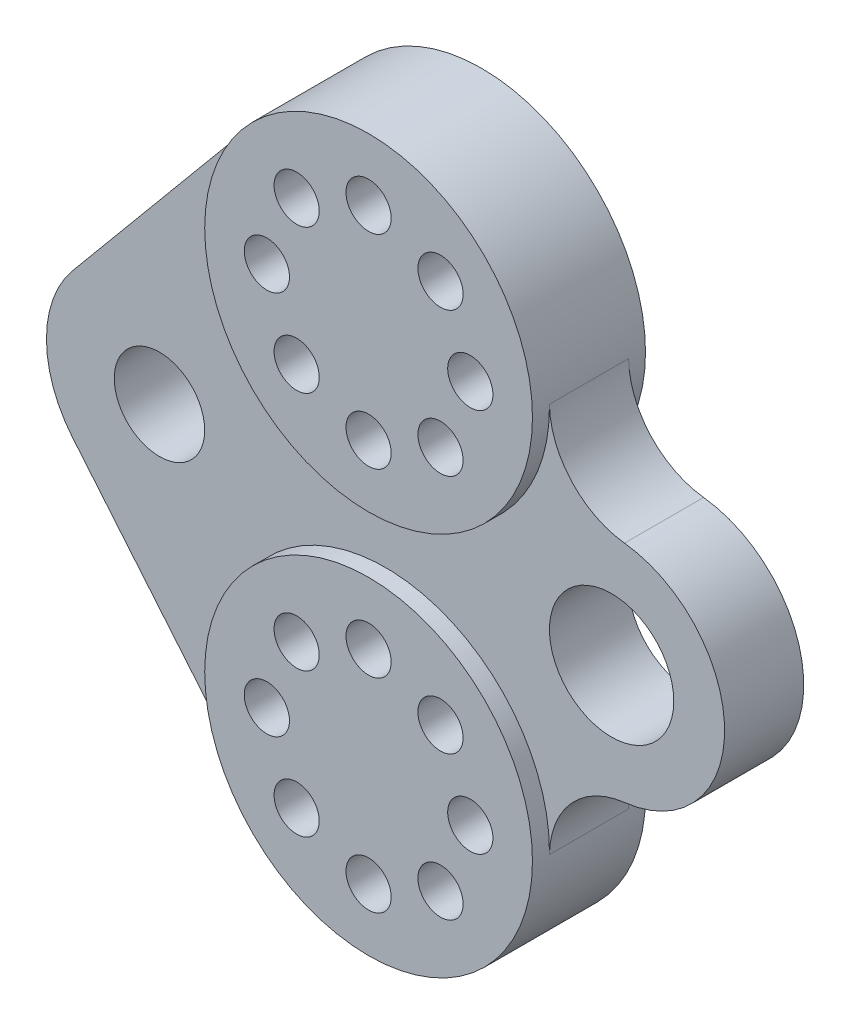
ISO-10303-21;
HEADER;
FILE_DESCRIPTION(('STEP AP214'),'2;1');
FILE_NAME('part.step','',(''),(''),'','','');
FILE_SCHEMA(('AUTOMOTIVE_DESIGN { 1 0 10303 214 1 1 1 1 }'));
ENDSEC;
DATA;
#1=APPLICATION_CONTEXT('core data for automotive mechanical design processes');
#2=APPLICATION_PROTOCOL_DEFINITION('international standard','automotive_design',2000,#1);
#3=PRODUCT_CONTEXT('',#1,'mechanical');
#4=PRODUCT('Part','Part','',(#3));
#5=PRODUCT_RELATED_PRODUCT_CATEGORY('part','',(#4));
#6=PRODUCT_DEFINITION_FORMATION('','',#4);
#7=PRODUCT_DEFINITION_CONTEXT('part definition',#1,'design');
#8=PRODUCT_DEFINITION('design','',#6,#7);
#9=PRODUCT_DEFINITION_SHAPE('','',#8);
#10=(LENGTH_UNIT() NAMED_UNIT(*) SI_UNIT(.MILLI.,.METRE.));
#11=(NAMED_UNIT(*) PLANE_ANGLE_UNIT() SI_UNIT($,.RADIAN.));
#12=(NAMED_UNIT(*) SI_UNIT($,.STERADIAN.) SOLID_ANGLE_UNIT());
#13=UNCERTAINTY_MEASURE_WITH_UNIT(LENGTH_MEASURE(1.E-05),#10,'distance_accuracy_value','');
#14=(GEOMETRIC_REPRESENTATION_CONTEXT(3) GLOBAL_UNCERTAINTY_ASSIGNED_CONTEXT((#13)) GLOBAL_UNIT_ASSIGNED_CONTEXT((#10,
#11,#12)) REPRESENTATION_CONTEXT('',''));
#15=CARTESIAN_POINT('',(0.,0.,0.));
#16=DIRECTION('',(0.,0.,1.));
#17=DIRECTION('',(1.,0.,0.));
#18=AXIS2_PLACEMENT_3D('',#15,#16,#17);
#19=CARTESIAN_POINT('',(-40.,-34.,7.));
#20=DIRECTION('',(0.,0.,1.));
#21=DIRECTION('',(1.,0.,0.));
#22=AXIS2_PLACEMENT_3D('',#19,#20,#21);
#23=PLANE('',#22);
#24=CARTESIAN_POINT('',(-40.,-34.,7.));
#25=DIRECTION('',(0.,0.,1.));
#26=DIRECTION('',(1.,0.,0.));
#27=AXIS2_PLACEMENT_3D('',#24,#25,#26);
#28=CIRCLE('',#27,8.00000000000001);
#29=CARTESIAN_POINT('',(-32.,-34.,7.));
#30=VERTEX_POINT('',#29);
#31=EDGE_CURVE('E141',#30,#30,#28,.T.);
#32=ORIENTED_EDGE('',*,*,#31,.F.);
#33=EDGE_LOOP('',(#32));
#34=FACE_BOUND('',#33,.T.);
#35=DIRECTION('',(0.639628478431684,-0.768684206666931,0.));
#36=VECTOR('',#35,1.);
#37=CARTESIAN_POINT('',(-55.3736841333386,-46.7925695686337,7.));
#38=LINE('',#37,#36);
#39=CARTESIAN_POINT('',(-55.3736841333386,-46.7925695686337,7.));
#40=VERTEX_POINT('',#39);
#41=CARTESIAN_POINT('',(-22.291841993341,-86.5492258745188,7.));
#42=VERTEX_POINT('',#41);
#43=EDGE_CURVE('E99',#40,#42,#38,.T.);
#44=ORIENTED_EDGE('',*,*,#43,.T.);
#45=CARTESIAN_POINT('',(0.,-68.,7.));
#46=DIRECTION('',(0.,0.,1.));
#47=DIRECTION('',(1.,0.,0.));
#48=AXIS2_PLACEMENT_3D('',#45,#46,#47);
#49=CIRCLE('',#48,29.);
#50=CARTESIAN_POINT('',(28.9955422378425,-68.5084587824885,7.));
#51=VERTEX_POINT('',#50);
#52=EDGE_CURVE('E168',#42,#51,#49,.F.);
#53=ORIENTED_EDGE('',*,*,#52,.T.);
#54=CARTESIAN_POINT('',(43.9932364987956,-68.7714547044654,7.));
#55=DIRECTION('',(0.,0.,-1.));
#56=DIRECTION('',(-1.,0.,0.));
#57=AXIS2_PLACEMENT_3D('',#54,#55,#56);
#58=CIRCLE('',#57,15.);
#59=CARTESIAN_POINT('',(42.2818494278832,-53.8694026882659,7.));
#60=VERTEX_POINT('',#59);
#61=EDGE_CURVE('E120',#51,#60,#58,.T.);
#62=ORIENTED_EDGE('',*,*,#61,.T.);
#63=CARTESIAN_POINT('',(40.,-34.,7.));
#64=DIRECTION('',(0.,0.,1.));
#65=DIRECTION('',(1.,0.,0.));
#66=AXIS2_PLACEMENT_3D('',#63,#64,#65);
#67=CIRCLE('',#66,20.);
#68=CARTESIAN_POINT('',(42.2818494278832,-14.1305973117341,7.));
#69=VERTEX_POINT('',#68);
#70=EDGE_CURVE('E112',#60,#69,#67,.T.);
#71=ORIENTED_EDGE('',*,*,#70,.T.);
#72=CARTESIAN_POINT('',(43.9932364987956,0.771454704465369,7.));
#73=DIRECTION('',(0.,0.,-1.));
#74=DIRECTION('',(1.,0.,0.));
#75=AXIS2_PLACEMENT_3D('',#72,#73,#74);
#76=CIRCLE('',#75,15.);
#77=CARTESIAN_POINT('',(28.9955422378425,0.508458782488539,7.));
#78=VERTEX_POINT('',#77);
#79=EDGE_CURVE('E113',#69,#78,#76,.T.);
#80=ORIENTED_EDGE('',*,*,#79,.T.);
#81=CARTESIAN_POINT('',(0.,0.,7.));
#82=DIRECTION('',(0.,0.,1.));
#83=DIRECTION('',(1.,0.,0.));
#84=AXIS2_PLACEMENT_3D('',#81,#82,#83);
#85=CIRCLE('',#84,29.);
#86=CARTESIAN_POINT('',(-22.291841993341,18.5492258745188,7.));
#87=VERTEX_POINT('',#86);
#88=EDGE_CURVE('E195',#78,#87,#85,.F.);
#89=ORIENTED_EDGE('',*,*,#88,.T.);
#90=DIRECTION('',(-0.639628478431684,-0.768684206666931,0.));
#91=VECTOR('',#90,1.);
#92=CARTESIAN_POINT('',(-55.3736841333386,-21.2074304313663,7.));
#93=LINE('',#92,#91);
#94=CARTESIAN_POINT('',(-55.3736841333386,-21.2074304313663,7.));
#95=VERTEX_POINT('',#94);
#96=EDGE_CURVE('E61',#87,#95,#93,.T.);
#97=ORIENTED_EDGE('',*,*,#96,.T.);
#98=CARTESIAN_POINT('',(-40.,-34.,7.));
#99=DIRECTION('',(0.,0.,1.));
#100=DIRECTION('',(1.,0.,0.));
#101=AXIS2_PLACEMENT_3D('',#98,#99,#100);
#102=CIRCLE('',#101,20.);
#103=EDGE_CURVE('E155',#95,#40,#102,.T.);
#104=ORIENTED_EDGE('',*,*,#103,.T.);
#105=EDGE_LOOP('',(#44,#53,#62,#71,#80,#89,#97,#104));
#106=FACE_BOUND('',#105,.T.);
#107=CARTESIAN_POINT('',(40.,-34.,7.));
#108=DIRECTION('',(0.,0.,1.));
#109=DIRECTION('',(1.,0.,0.));
#110=AXIS2_PLACEMENT_3D('',#107,#108,#109);
#111=CIRCLE('',#110,11.);
#112=CARTESIAN_POINT('',(51.,-34.,7.));
#113=VERTEX_POINT('',#112);
#114=EDGE_CURVE('E189',#113,#113,#111,.T.);
#115=ORIENTED_EDGE('',*,*,#114,.F.);
#116=EDGE_LOOP('',(#115));
#117=FACE_BOUND('',#116,.T.);
#118=ADVANCED_FACE('F44',(#34,#106,#117),#23,.T.);
#119=CARTESIAN_POINT('',(-40.,-34.,-7.));
#120=DIRECTION('',(0.,0.,1.));
#121=DIRECTION('',(1.,0.,0.));
#122=AXIS2_PLACEMENT_3D('',#119,#120,#121);
#123=PLANE('',#122);
#124=CARTESIAN_POINT('',(0.,-68.,-7.));
#125=DIRECTION('',(0.,0.,1.));
#126=DIRECTION('',(1.,0.,0.));
#127=AXIS2_PLACEMENT_3D('',#124,#125,#126);
#128=CIRCLE('',#127,29.);
#129=CARTESIAN_POINT('',(-22.291841993341,-86.5492258745188,-7.));
#130=VERTEX_POINT('',#129);
#131=CARTESIAN_POINT('',(28.9955422378425,-68.5084587824885,-7.));
#132=VERTEX_POINT('',#131);
#133=EDGE_CURVE('E169',#130,#132,#128,.F.);
#134=ORIENTED_EDGE('',*,*,#133,.F.);
#135=DIRECTION('',(0.639628478431684,-0.768684206666931,0.));
#136=VECTOR('',#135,1.);
#137=CARTESIAN_POINT('',(-55.3736841333386,-46.7925695686337,-7.));
#138=LINE('',#137,#136);
#139=CARTESIAN_POINT('',(-55.3736841333386,-46.7925695686337,-7.));
#140=VERTEX_POINT('',#139);
#141=EDGE_CURVE('E142',#140,#130,#138,.T.);
#142=ORIENTED_EDGE('',*,*,#141,.F.);
#143=CARTESIAN_POINT('',(-40.,-34.,-7.));
#144=DIRECTION('',(0.,0.,1.));
#145=DIRECTION('',(1.,0.,0.));
#146=AXIS2_PLACEMENT_3D('',#143,#144,#145);
#147=CIRCLE('',#146,20.);
#148=CARTESIAN_POINT('',(-55.3736841333386,-21.2074304313663,-7.));
#149=VERTEX_POINT('',#148);
#150=EDGE_CURVE('E139',#149,#140,#147,.T.);
#151=ORIENTED_EDGE('',*,*,#150,.F.);
#152=DIRECTION('',(-0.639628478431684,-0.768684206666931,0.));
#153=VECTOR('',#152,1.);
#154=CARTESIAN_POINT('',(-55.3736841333386,-21.2074304313663,-7.));
#155=LINE('',#154,#153);
#156=CARTESIAN_POINT('',(-22.291841993341,18.5492258745188,-7.));
#157=VERTEX_POINT('',#156);
#158=EDGE_CURVE('E95',#157,#149,#155,.T.);
#159=ORIENTED_EDGE('',*,*,#158,.F.);
#160=CARTESIAN_POINT('',(0.,0.,-7.));
#161=DIRECTION('',(0.,0.,1.));
#162=DIRECTION('',(1.,0.,0.));
#163=AXIS2_PLACEMENT_3D('',#160,#161,#162);
#164=CIRCLE('',#163,29.);
#165=CARTESIAN_POINT('',(28.9955422378425,0.508458782488539,-7.));
#166=VERTEX_POINT('',#165);
#167=EDGE_CURVE('E88',#166,#157,#164,.F.);
#168=ORIENTED_EDGE('',*,*,#167,.F.);
#169=CARTESIAN_POINT('',(43.9932364987956,0.771454704465369,-7.));
#170=DIRECTION('',(0.,0.,-1.));
#171=DIRECTION('',(1.,0.,0.));
#172=AXIS2_PLACEMENT_3D('',#169,#170,#171);
#173=CIRCLE('',#172,15.);
#174=CARTESIAN_POINT('',(42.2818494278832,-14.1305973117341,-7.));
#175=VERTEX_POINT('',#174);
#176=EDGE_CURVE('E149',#175,#166,#173,.T.);
#177=ORIENTED_EDGE('',*,*,#176,.F.);
#178=CARTESIAN_POINT('',(40.,-34.,-7.));
#179=DIRECTION('',(0.,0.,1.));
#180=DIRECTION('',(1.,0.,0.));
#181=AXIS2_PLACEMENT_3D('',#178,#179,#180);
#182=CIRCLE('',#181,20.);
#183=CARTESIAN_POINT('',(42.2818494278832,-53.8694026882659,-7.));
#184=VERTEX_POINT('',#183);
#185=EDGE_CURVE('E130',#184,#175,#182,.T.);
#186=ORIENTED_EDGE('',*,*,#185,.F.);
#187=CARTESIAN_POINT('',(43.9932364987956,-68.7714547044654,-7.));
#188=DIRECTION('',(0.,0.,-1.));
#189=DIRECTION('',(-1.,0.,0.));
#190=AXIS2_PLACEMENT_3D('',#187,#188,#189);
#191=CIRCLE('',#190,15.);
#192=EDGE_CURVE('E148',#132,#184,#191,.T.);
#193=ORIENTED_EDGE('',*,*,#192,.F.);
#194=EDGE_LOOP('',(#134,#142,#151,#159,#168,#177,#186,#193));
#195=FACE_BOUND('',#194,.T.);
#196=CARTESIAN_POINT('',(-40.,-34.,-7.));
#197=DIRECTION('',(0.,0.,1.));
#198=DIRECTION('',(1.,0.,0.));
#199=AXIS2_PLACEMENT_3D('',#196,#197,#198);
#200=CIRCLE('',#199,8.00000000000001);
#201=CARTESIAN_POINT('',(-32.,-34.,-7.));
#202=VERTEX_POINT('',#201);
#203=EDGE_CURVE('E181',#202,#202,#200,.T.);
#204=ORIENTED_EDGE('',*,*,#203,.T.);
#205=EDGE_LOOP('',(#204));
#206=FACE_BOUND('',#205,.T.);
#207=CARTESIAN_POINT('',(40.,-34.,-7.));
#208=DIRECTION('',(0.,0.,1.));
#209=DIRECTION('',(1.,0.,0.));
#210=AXIS2_PLACEMENT_3D('',#207,#208,#209);
#211=CIRCLE('',#210,11.);
#212=CARTESIAN_POINT('',(51.,-34.,-7.));
#213=VERTEX_POINT('',#212);
#214=EDGE_CURVE('E188',#213,#213,#211,.T.);
#215=ORIENTED_EDGE('',*,*,#214,.T.);
#216=EDGE_LOOP('',(#215));
#217=FACE_BOUND('',#216,.T.);
#218=ADVANCED_FACE('F178',(#195,#206,#217),#123,.F.);
#219=CARTESIAN_POINT('',(-40.,-34.,7.));
#220=DIRECTION('',(0.,0.,-1.));
#221=DIRECTION('',(-1.,0.,0.));
#222=AXIS2_PLACEMENT_3D('',#219,#220,#221);
#223=CYLINDRICAL_SURFACE('',#222,20.);
#224=ORIENTED_EDGE('',*,*,#150,.T.);
#225=DIRECTION('',(0.,0.,-1.));
#226=VECTOR('',#225,1.);
#227=CARTESIAN_POINT('',(-55.3736841333386,-46.7925695686337,7.));
#228=LINE('',#227,#226);
#229=EDGE_CURVE('E11',#40,#140,#228,.T.);
#230=ORIENTED_EDGE('',*,*,#229,.F.);
#231=ORIENTED_EDGE('',*,*,#103,.F.);
#232=DIRECTION('',(0.,0.,-1.));
#233=VECTOR('',#232,1.);
#234=CARTESIAN_POINT('',(-55.3736841333386,-21.2074304313663,7.));
#235=LINE('',#234,#233);
#236=EDGE_CURVE('E132',#95,#149,#235,.T.);
#237=ORIENTED_EDGE('',*,*,#236,.T.);
#238=EDGE_LOOP('',(#224,#230,#231,#237));
#239=FACE_BOUND('',#238,.T.);
#240=ADVANCED_FACE('F50',(#239),#223,.T.);
#241=CARTESIAN_POINT('',(-55.3736841333386,-46.7925695686337,7.));
#242=DIRECTION('',(0.768684206666931,0.639628478431684,0.));
#243=DIRECTION('',(-0.639628478431684,0.768684206666931,0.));
#244=AXIS2_PLACEMENT_3D('',#241,#242,#243);
#245=PLANE('',#244);
#246=ORIENTED_EDGE('',*,*,#141,.T.);
#247=DIRECTION('',(0.,0.,-1.));
#248=VECTOR('',#247,1.);
#249=CARTESIAN_POINT('',(-22.291841993341,-86.5492258745188,7.));
#250=LINE('',#249,#248);
#251=EDGE_CURVE('E53',#42,#130,#250,.T.);
#252=ORIENTED_EDGE('',*,*,#251,.F.);
#253=ORIENTED_EDGE('',*,*,#43,.F.);
#254=ORIENTED_EDGE('',*,*,#229,.T.);
#255=EDGE_LOOP('',(#246,#252,#253,#254));
#256=FACE_BOUND('',#255,.T.);
#257=ADVANCED_FACE('F174',(#256),#245,.F.);
#258=CARTESIAN_POINT('',(0.,-68.,7.));
#259=DIRECTION('',(0.,0.,-1.));
#260=DIRECTION('',(-1.,0.,0.));
#261=AXIS2_PLACEMENT_3D('',#258,#259,#260);
#262=CYLINDRICAL_SURFACE('',#261,29.);
#263=ORIENTED_EDGE('',*,*,#251,.T.);
#264=ORIENTED_EDGE('',*,*,#133,.T.);
#265=DIRECTION('',(0.,0.,-1.));
#266=VECTOR('',#265,1.);
#267=CARTESIAN_POINT('',(28.9955422378425,-68.5084587824885,7.));
#268=LINE('',#267,#266);
#269=EDGE_CURVE('E158',#51,#132,#268,.T.);
#270=ORIENTED_EDGE('',*,*,#269,.F.);
#271=ORIENTED_EDGE('',*,*,#52,.F.);
#272=EDGE_LOOP('',(#263,#264,#270,#271));
#273=FACE_BOUND('',#272,.T.);
#274=CARTESIAN_POINT('',(0.,-68.,-10.));
#275=DIRECTION('',(0.,0.,1.));
#276=DIRECTION('',(1.,0.,0.));
#277=AXIS2_PLACEMENT_3D('',#274,#275,#276);
#278=CIRCLE('',#277,29.);
#279=CARTESIAN_POINT('',(29.,-68.,-10.));
#280=VERTEX_POINT('',#279);
#281=EDGE_CURVE('E206',#280,#280,#278,.T.);
#282=ORIENTED_EDGE('',*,*,#281,.T.);
#283=EDGE_LOOP('',(#282));
#284=FACE_BOUND('',#283,.T.);
#285=CARTESIAN_POINT('',(0.,-68.,10.));
#286=DIRECTION('',(0.,0.,1.));
#287=DIRECTION('',(1.,0.,0.));
#288=AXIS2_PLACEMENT_3D('',#285,#286,#287);
#289=CIRCLE('',#288,29.);
#290=CARTESIAN_POINT('',(29.,-68.,10.));
#291=VERTEX_POINT('',#290);
#292=EDGE_CURVE('E202',#291,#291,#289,.T.);
#293=ORIENTED_EDGE('',*,*,#292,.F.);
#294=EDGE_LOOP('',(#293));
#295=FACE_BOUND('',#294,.T.);
#296=ADVANCED_FACE('F163',(#273,#284,#295),#262,.T.);
#297=CARTESIAN_POINT('',(43.9932364987956,-68.7714547044654,7.));
#298=DIRECTION('',(0.,0.,-1.));
#299=DIRECTION('',(-1.,0.,0.));
#300=AXIS2_PLACEMENT_3D('',#297,#298,#299);
#301=CYLINDRICAL_SURFACE('',#300,15.);
#302=ORIENTED_EDGE('',*,*,#192,.T.);
#303=DIRECTION('',(0.,0.,-1.));
#304=VECTOR('',#303,1.);
#305=CARTESIAN_POINT('',(42.2818494278832,-53.8694026882659,7.));
#306=LINE('',#305,#304);
#307=EDGE_CURVE('E129',#60,#184,#306,.T.);
#308=ORIENTED_EDGE('',*,*,#307,.F.);
#309=ORIENTED_EDGE('',*,*,#61,.F.);
#310=ORIENTED_EDGE('',*,*,#269,.T.);
#311=EDGE_LOOP('',(#302,#308,#309,#310));
#312=FACE_BOUND('',#311,.T.);
#313=ADVANCED_FACE('F179',(#312),#301,.F.);
#314=CARTESIAN_POINT('',(40.,-34.,7.));
#315=DIRECTION('',(0.,0.,-1.));
#316=DIRECTION('',(-1.,0.,0.));
#317=AXIS2_PLACEMENT_3D('',#314,#315,#316);
#318=CYLINDRICAL_SURFACE('',#317,20.);
#319=ORIENTED_EDGE('',*,*,#185,.T.);
#320=DIRECTION('',(0.,0.,-1.));
#321=VECTOR('',#320,1.);
#322=CARTESIAN_POINT('',(42.2818494278832,-14.1305973117341,7.));
#323=LINE('',#322,#321);
#324=EDGE_CURVE('E124',#69,#175,#323,.T.);
#325=ORIENTED_EDGE('',*,*,#324,.F.);
#326=ORIENTED_EDGE('',*,*,#70,.F.);
#327=ORIENTED_EDGE('',*,*,#307,.T.);
#328=EDGE_LOOP('',(#319,#325,#326,#327));
#329=FACE_BOUND('',#328,.T.);
#330=ADVANCED_FACE('F122',(#329),#318,.T.);
#331=CARTESIAN_POINT('',(43.9932364987956,0.771454704465369,7.));
#332=DIRECTION('',(0.,0.,-1.));
#333=DIRECTION('',(-1.,0.,0.));
#334=AXIS2_PLACEMENT_3D('',#331,#332,#333);
#335=CYLINDRICAL_SURFACE('',#334,15.);
#336=ORIENTED_EDGE('',*,*,#176,.T.);
#337=DIRECTION('',(0.,0.,-1.));
#338=VECTOR('',#337,1.);
#339=CARTESIAN_POINT('',(28.9955422378425,0.508458782488539,7.));
#340=LINE('',#339,#338);
#341=EDGE_CURVE('E128',#78,#166,#340,.T.);
#342=ORIENTED_EDGE('',*,*,#341,.F.);
#343=ORIENTED_EDGE('',*,*,#79,.F.);
#344=ORIENTED_EDGE('',*,*,#324,.T.);
#345=EDGE_LOOP('',(#336,#342,#343,#344));
#346=FACE_BOUND('',#345,.T.);
#347=ADVANCED_FACE('F131',(#346),#335,.F.);
#348=CARTESIAN_POINT('',(0.,0.,7.));
#349=DIRECTION('',(0.,0.,-1.));
#350=DIRECTION('',(-1.,0.,0.));
#351=AXIS2_PLACEMENT_3D('',#348,#349,#350);
#352=CYLINDRICAL_SURFACE('',#351,29.);
#353=ORIENTED_EDGE('',*,*,#341,.T.);
#354=ORIENTED_EDGE('',*,*,#167,.T.);
#355=DIRECTION('',(0.,0.,-1.));
#356=VECTOR('',#355,1.);
#357=CARTESIAN_POINT('',(-22.291841993341,18.5492258745188,7.));
#358=LINE('',#357,#356);
#359=EDGE_CURVE('E152',#87,#157,#358,.T.);
#360=ORIENTED_EDGE('',*,*,#359,.F.);
#361=ORIENTED_EDGE('',*,*,#88,.F.);
#362=EDGE_LOOP('',(#353,#354,#360,#361));
#363=FACE_BOUND('',#362,.T.);
#364=CARTESIAN_POINT('',(0.,0.,-10.));
#365=DIRECTION('',(0.,0.,1.));
#366=DIRECTION('',(1.,0.,0.));
#367=AXIS2_PLACEMENT_3D('',#364,#365,#366);
#368=CIRCLE('',#367,29.);
#369=CARTESIAN_POINT('',(29.,0.,-10.));
#370=VERTEX_POINT('',#369);
#371=EDGE_CURVE('E196',#370,#370,#368,.T.);
#372=ORIENTED_EDGE('',*,*,#371,.T.);
#373=EDGE_LOOP('',(#372));
#374=FACE_BOUND('',#373,.T.);
#375=CARTESIAN_POINT('',(0.,0.,10.));
#376=DIRECTION('',(0.,0.,1.));
#377=DIRECTION('',(1.,0.,0.));
#378=AXIS2_PLACEMENT_3D('',#375,#376,#377);
#379=CIRCLE('',#378,29.);
#380=CARTESIAN_POINT('',(29.,0.,10.));
#381=VERTEX_POINT('',#380);
#382=EDGE_CURVE('E197',#381,#381,#379,.T.);
#383=ORIENTED_EDGE('',*,*,#382,.F.);
#384=EDGE_LOOP('',(#383));
#385=FACE_BOUND('',#384,.T.);
#386=ADVANCED_FACE('F334',(#363,#374,#385),#352,.T.);
#387=CARTESIAN_POINT('',(-55.3736841333386,-21.2074304313663,7.));
#388=DIRECTION('',(0.768684206666931,-0.639628478431684,0.));
#389=DIRECTION('',(0.639628478431684,0.768684206666931,0.));
#390=AXIS2_PLACEMENT_3D('',#387,#388,#389);
#391=PLANE('',#390);
#392=ORIENTED_EDGE('',*,*,#158,.T.);
#393=ORIENTED_EDGE('',*,*,#236,.F.);
#394=ORIENTED_EDGE('',*,*,#96,.F.);
#395=ORIENTED_EDGE('',*,*,#359,.T.);
#396=EDGE_LOOP('',(#392,#393,#394,#395));
#397=FACE_BOUND('',#396,.T.);
#398=ADVANCED_FACE('F333',(#397),#391,.F.);
#399=CARTESIAN_POINT('',(-40.,-34.,7.));
#400=DIRECTION('',(0.,0.,-1.));
#401=DIRECTION('',(-1.,0.,0.));
#402=AXIS2_PLACEMENT_3D('',#399,#400,#401);
#403=CYLINDRICAL_SURFACE('',#402,8.00000000000001);
#404=ORIENTED_EDGE('',*,*,#31,.T.);
#405=EDGE_LOOP('',(#404));
#406=FACE_BOUND('',#405,.T.);
#407=ORIENTED_EDGE('',*,*,#203,.F.);
#408=EDGE_LOOP('',(#407));
#409=FACE_BOUND('',#408,.T.);
#410=ADVANCED_FACE('F345',(#406,#409),#403,.F.);
#411=CARTESIAN_POINT('',(40.,-34.,7.));
#412=DIRECTION('',(0.,0.,-1.));
#413=DIRECTION('',(-1.,0.,0.));
#414=AXIS2_PLACEMENT_3D('',#411,#412,#413);
#415=CYLINDRICAL_SURFACE('',#414,11.);
#416=ORIENTED_EDGE('',*,*,#114,.T.);
#417=EDGE_LOOP('',(#416));
#418=FACE_BOUND('',#417,.T.);
#419=ORIENTED_EDGE('',*,*,#214,.F.);
#420=EDGE_LOOP('',(#419));
#421=FACE_BOUND('',#420,.T.);
#422=ADVANCED_FACE('F356',(#418,#421),#415,.F.);
#423=CARTESIAN_POINT('',(0.,0.,-10.));
#424=DIRECTION('',(0.,0.,1.));
#425=DIRECTION('',(1.,0.,0.));
#426=AXIS2_PLACEMENT_3D('',#423,#424,#425);
#427=PLANE('',#426);
#428=CARTESIAN_POINT('',(0.,18.,-10.));
#429=DIRECTION('',(0.,0.,1.));
#430=DIRECTION('',(1.,0.,0.));
#431=AXIS2_PLACEMENT_3D('',#428,#429,#430);
#432=CIRCLE('',#431,4.);
#433=CARTESIAN_POINT('',(4.,18.,-10.));
#434=VERTEX_POINT('',#433);
#435=EDGE_CURVE('E214',#434,#434,#432,.T.);
#436=ORIENTED_EDGE('',*,*,#435,.T.);
#437=EDGE_LOOP('',(#436));
#438=FACE_BOUND('',#437,.T.);
#439=CARTESIAN_POINT('',(12.7279220613581,12.7279220613584,-10.));
#440=DIRECTION('',(0.,0.,1.));
#441=DIRECTION('',(1.,0.,0.));
#442=AXIS2_PLACEMENT_3D('',#439,#440,#441);
#443=CIRCLE('',#442,4.00000000000009);
#444=CARTESIAN_POINT('',(16.7279220613582,12.7279220613584,-10.));
#445=VERTEX_POINT('',#444);
#446=EDGE_CURVE('E280',#445,#445,#443,.T.);
#447=ORIENTED_EDGE('',*,*,#446,.T.);
#448=EDGE_LOOP('',(#447));
#449=FACE_BOUND('',#448,.T.);
#450=CARTESIAN_POINT('',(18.0000000000008,7.6407960826321E-13,-10.));
#451=DIRECTION('',(0.,0.,1.));
#452=DIRECTION('',(1.,0.,0.));
#453=AXIS2_PLACEMENT_3D('',#450,#451,#452);
#454=CIRCLE('',#453,4.00000000000057);
#455=CARTESIAN_POINT('',(22.0000000000013,7.6407960826321E-13,-10.));
#456=VERTEX_POINT('',#455);
#457=EDGE_CURVE('E271',#456,#456,#454,.T.);
#458=ORIENTED_EDGE('',*,*,#457,.T.);
#459=EDGE_LOOP('',(#458));
#460=FACE_BOUND('',#459,.T.);
#461=CARTESIAN_POINT('',(12.7279220613592,-12.7279220613573,-10.));
#462=DIRECTION('',(0.,0.,1.));
#463=DIRECTION('',(1.,0.,0.));
#464=AXIS2_PLACEMENT_3D('',#461,#462,#463);
#465=CIRCLE('',#464,4.00000000000118);
#466=CARTESIAN_POINT('',(16.7279220613603,-12.7279220613573,-10.));
#467=VERTEX_POINT('',#466);
#468=EDGE_CURVE('E262',#467,#467,#465,.T.);
#469=ORIENTED_EDGE('',*,*,#468,.T.);
#470=EDGE_LOOP('',(#469));
#471=FACE_BOUND('',#470,.T.);
#472=CARTESIAN_POINT('',(1.52815921652642E-12,-18.,-10.));
#473=DIRECTION('',(0.,0.,1.));
#474=DIRECTION('',(1.,0.,0.));
#475=AXIS2_PLACEMENT_3D('',#472,#473,#474);
#476=CIRCLE('',#475,4.00000000000158);
#477=CARTESIAN_POINT('',(4.00000000000311,-18.,-10.));
#478=VERTEX_POINT('',#477);
#479=EDGE_CURVE('E264',#478,#478,#476,.T.);
#480=ORIENTED_EDGE('',*,*,#479,.T.);
#481=EDGE_LOOP('',(#480));
#482=FACE_BOUND('',#481,.T.);
#483=CARTESIAN_POINT('',(-12.7279220613566,-12.7279220613584,-10.));
#484=DIRECTION('',(0.,0.,1.));
#485=DIRECTION('',(1.,0.,0.));
#486=AXIS2_PLACEMENT_3D('',#483,#484,#485);
#487=CIRCLE('',#486,4.00000000000156);
#488=CARTESIAN_POINT('',(-8.727922061355,-12.7279220613584,-10.));
#489=VERTEX_POINT('',#488);
#490=EDGE_CURVE('E298',#489,#489,#487,.T.);
#491=ORIENTED_EDGE('',*,*,#490,.T.);
#492=EDGE_LOOP('',(#491));
#493=FACE_BOUND('',#492,.T.);
#494=CARTESIAN_POINT('',(-17.9999999999992,-7.66283972501675E-13,-10.));
#495=DIRECTION('',(0.,0.,1.));
#496=DIRECTION('',(1.,0.,0.));
#497=AXIS2_PLACEMENT_3D('',#494,#495,#496);
#498=CIRCLE('',#497,4.00000000000114);
#499=CARTESIAN_POINT('',(-13.9999999999981,-7.66283972501675E-13,-10.));
#500=VERTEX_POINT('',#499);
#501=EDGE_CURVE('E291',#500,#500,#498,.T.);
#502=ORIENTED_EDGE('',*,*,#501,.T.);
#503=EDGE_LOOP('',(#502));
#504=FACE_BOUND('',#503,.T.);
#505=CARTESIAN_POINT('',(-12.7279220613576,12.7279220613573,-10.));
#506=DIRECTION('',(0.,0.,1.));
#507=DIRECTION('',(1.,0.,0.));
#508=AXIS2_PLACEMENT_3D('',#505,#506,#507);
#509=CIRCLE('',#508,4.00000000000059);
#510=CARTESIAN_POINT('',(-8.72792206135705,12.7279220613573,-10.));
#511=VERTEX_POINT('',#510);
#512=EDGE_CURVE('E290',#511,#511,#509,.T.);
#513=ORIENTED_EDGE('',*,*,#512,.T.);
#514=EDGE_LOOP('',(#513));
#515=FACE_BOUND('',#514,.T.);
#516=ORIENTED_EDGE('',*,*,#371,.F.);
#517=EDGE_LOOP('',(#516));
#518=FACE_BOUND('',#517,.T.);
#519=ADVANCED_FACE('F306',(#438,#449,#460,#471,#482,#493,#504,#515,#518),#427,.F.);
#520=CARTESIAN_POINT('',(0.,0.,10.));
#521=DIRECTION('',(0.,0.,1.));
#522=DIRECTION('',(1.,0.,0.));
#523=AXIS2_PLACEMENT_3D('',#520,#521,#522);
#524=PLANE('',#523);
#525=CARTESIAN_POINT('',(0.,18.,10.));
#526=DIRECTION('',(0.,0.,1.));
#527=DIRECTION('',(1.,0.,0.));
#528=AXIS2_PLACEMENT_3D('',#525,#526,#527);
#529=CIRCLE('',#528,4.);
#530=CARTESIAN_POINT('',(4.,18.,10.));
#531=VERTEX_POINT('',#530);
#532=EDGE_CURVE('E278',#531,#531,#529,.T.);
#533=ORIENTED_EDGE('',*,*,#532,.F.);
#534=EDGE_LOOP('',(#533));
#535=FACE_BOUND('',#534,.T.);
#536=CARTESIAN_POINT('',(12.7279220613581,12.7279220613584,10.));
#537=DIRECTION('',(0.,0.,1.));
#538=DIRECTION('',(1.,0.,0.));
#539=AXIS2_PLACEMENT_3D('',#536,#537,#538);
#540=CIRCLE('',#539,4.00000000000009);
#541=CARTESIAN_POINT('',(16.7279220613582,12.7279220613584,10.));
#542=VERTEX_POINT('',#541);
#543=EDGE_CURVE('E273',#542,#542,#540,.T.);
#544=ORIENTED_EDGE('',*,*,#543,.F.);
#545=EDGE_LOOP('',(#544));
#546=FACE_BOUND('',#545,.T.);
#547=CARTESIAN_POINT('',(18.0000000000008,7.6407960826321E-13,10.));
#548=DIRECTION('',(0.,0.,1.));
#549=DIRECTION('',(1.,0.,0.));
#550=AXIS2_PLACEMENT_3D('',#547,#548,#549);
#551=CIRCLE('',#550,4.00000000000057);
#552=CARTESIAN_POINT('',(22.0000000000013,7.6407960826321E-13,10.));
#553=VERTEX_POINT('',#552);
#554=EDGE_CURVE('E268',#553,#553,#551,.T.);
#555=ORIENTED_EDGE('',*,*,#554,.F.);
#556=EDGE_LOOP('',(#555));
#557=FACE_BOUND('',#556,.T.);
#558=CARTESIAN_POINT('',(12.7279220613592,-12.7279220613573,10.));
#559=DIRECTION('',(0.,0.,1.));
#560=DIRECTION('',(1.,0.,0.));
#561=AXIS2_PLACEMENT_3D('',#558,#559,#560);
#562=CIRCLE('',#561,4.00000000000118);
#563=CARTESIAN_POINT('',(16.7279220613603,-12.7279220613573,10.));
#564=VERTEX_POINT('',#563);
#565=EDGE_CURVE('E261',#564,#564,#562,.T.);
#566=ORIENTED_EDGE('',*,*,#565,.F.);
#567=EDGE_LOOP('',(#566));
#568=FACE_BOUND('',#567,.T.);
#569=CARTESIAN_POINT('',(1.52815921652642E-12,-18.,10.));
#570=DIRECTION('',(0.,0.,1.));
#571=DIRECTION('',(1.,0.,0.));
#572=AXIS2_PLACEMENT_3D('',#569,#570,#571);
#573=CIRCLE('',#572,4.00000000000158);
#574=CARTESIAN_POINT('',(4.00000000000311,-18.,10.));
#575=VERTEX_POINT('',#574);
#576=EDGE_CURVE('E305',#575,#575,#573,.T.);
#577=ORIENTED_EDGE('',*,*,#576,.F.);
#578=EDGE_LOOP('',(#577));
#579=FACE_BOUND('',#578,.T.);
#580=CARTESIAN_POINT('',(-12.7279220613566,-12.7279220613584,10.));
#581=DIRECTION('',(0.,0.,1.));
#582=DIRECTION('',(1.,0.,0.));
#583=AXIS2_PLACEMENT_3D('',#580,#581,#582);
#584=CIRCLE('',#583,4.00000000000156);
#585=CARTESIAN_POINT('',(-8.727922061355,-12.7279220613584,10.));
#586=VERTEX_POINT('',#585);
#587=EDGE_CURVE('E299',#586,#586,#584,.T.);
#588=ORIENTED_EDGE('',*,*,#587,.F.);
#589=EDGE_LOOP('',(#588));
#590=FACE_BOUND('',#589,.T.);
#591=CARTESIAN_POINT('',(-17.9999999999992,-7.66283972501675E-13,10.));
#592=DIRECTION('',(0.,0.,1.));
#593=DIRECTION('',(1.,0.,0.));
#594=AXIS2_PLACEMENT_3D('',#591,#592,#593);
#595=CIRCLE('',#594,4.00000000000114);
#596=CARTESIAN_POINT('',(-13.9999999999981,-7.66283972501675E-13,10.));
#597=VERTEX_POINT('',#596);
#598=EDGE_CURVE('E287',#597,#597,#595,.T.);
#599=ORIENTED_EDGE('',*,*,#598,.F.);
#600=EDGE_LOOP('',(#599));
#601=FACE_BOUND('',#600,.T.);
#602=CARTESIAN_POINT('',(-12.7279220613576,12.7279220613573,10.));
#603=DIRECTION('',(0.,0.,1.));
#604=DIRECTION('',(1.,0.,0.));
#605=AXIS2_PLACEMENT_3D('',#602,#603,#604);
#606=CIRCLE('',#605,4.00000000000059);
#607=CARTESIAN_POINT('',(-8.72792206135705,12.7279220613573,10.));
#608=VERTEX_POINT('',#607);
#609=EDGE_CURVE('E257',#608,#608,#606,.T.);
#610=ORIENTED_EDGE('',*,*,#609,.F.);
#611=EDGE_LOOP('',(#610));
#612=FACE_BOUND('',#611,.T.);
#613=ORIENTED_EDGE('',*,*,#382,.T.);
#614=EDGE_LOOP('',(#613));
#615=FACE_BOUND('',#614,.T.);
#616=ADVANCED_FACE('F317',(#535,#546,#557,#568,#579,#590,#601,#612,#615),#524,.T.);
#617=CARTESIAN_POINT('',(0.,-68.,-10.));
#618=DIRECTION('',(0.,0.,1.));
#619=DIRECTION('',(1.,0.,0.));
#620=AXIS2_PLACEMENT_3D('',#617,#618,#619);
#621=PLANE('',#620);
#622=CARTESIAN_POINT('',(-12.7279220613576,-55.2720779386423,-10.));
#623=DIRECTION('',(0.,0.,1.));
#624=DIRECTION('',(1.,0.,0.));
#625=AXIS2_PLACEMENT_3D('',#622,#623,#624);
#626=CIRCLE('',#625,3.99999999999999);
#627=CARTESIAN_POINT('',(-8.72792206135757,-55.2720779386423,-10.));
#628=VERTEX_POINT('',#627);
#629=EDGE_CURVE('E222',#628,#628,#626,.T.);
#630=ORIENTED_EDGE('',*,*,#629,.T.);
#631=EDGE_LOOP('',(#630));
#632=FACE_BOUND('',#631,.T.);
#633=CARTESIAN_POINT('',(-17.9999999999995,-68.0000000000003,-10.));
#634=DIRECTION('',(0.,0.,1.));
#635=DIRECTION('',(1.,0.,0.));
#636=AXIS2_PLACEMENT_3D('',#633,#634,#635);
#637=CIRCLE('',#636,4.00000000000001);
#638=CARTESIAN_POINT('',(-13.9999999999995,-68.0000000000003,-10.));
#639=VERTEX_POINT('',#638);
#640=EDGE_CURVE('E226',#639,#639,#637,.T.);
#641=ORIENTED_EDGE('',*,*,#640,.T.);
#642=EDGE_LOOP('',(#641));
#643=FACE_BOUND('',#642,.T.);
#644=CARTESIAN_POINT('',(-12.7279220613571,-80.7279220613581,-10.));
#645=DIRECTION('',(0.,0.,1.));
#646=DIRECTION('',(1.,0.,0.));
#647=AXIS2_PLACEMENT_3D('',#644,#645,#646);
#648=CIRCLE('',#647,4.00000000000001);
#649=CARTESIAN_POINT('',(-8.72792206135708,-80.7279220613581,-10.));
#650=VERTEX_POINT('',#649);
#651=EDGE_CURVE('E231',#650,#650,#648,.T.);
#652=ORIENTED_EDGE('',*,*,#651,.T.);
#653=EDGE_LOOP('',(#652));
#654=FACE_BOUND('',#653,.T.);
#655=CARTESIAN_POINT('',(8.88670754342331E-13,-86.,-10.));
#656=DIRECTION('',(0.,0.,1.));
#657=DIRECTION('',(1.,0.,0.));
#658=AXIS2_PLACEMENT_3D('',#655,#656,#657);
#659=CIRCLE('',#658,4.);
#660=CARTESIAN_POINT('',(4.00000000000089,-86.,-10.));
#661=VERTEX_POINT('',#660);
#662=EDGE_CURVE('E239',#661,#661,#659,.T.);
#663=ORIENTED_EDGE('',*,*,#662,.T.);
#664=EDGE_LOOP('',(#663));
#665=FACE_BOUND('',#664,.T.);
#666=CARTESIAN_POINT('',(12.7279220613587,-80.7279220613576,-10.));
#667=DIRECTION('',(0.,0.,1.));
#668=DIRECTION('',(1.,0.,0.));
#669=AXIS2_PLACEMENT_3D('',#666,#667,#668);
#670=CIRCLE('',#669,4.00000000000001);
#671=CARTESIAN_POINT('',(16.7279220613587,-80.7279220613576,-10.));
#672=VERTEX_POINT('',#671);
#673=EDGE_CURVE('E242',#672,#672,#670,.T.);
#674=ORIENTED_EDGE('',*,*,#673,.T.);
#675=EDGE_LOOP('',(#674));
#676=FACE_BOUND('',#675,.T.);
#677=CARTESIAN_POINT('',(18.0000000000005,-67.9999999999995,-10.));
#678=DIRECTION('',(0.,0.,1.));
#679=DIRECTION('',(1.,0.,0.));
#680=AXIS2_PLACEMENT_3D('',#677,#678,#679);
#681=CIRCLE('',#680,4.);
#682=CARTESIAN_POINT('',(22.0000000000005,-67.9999999999995,-10.));
#683=VERTEX_POINT('',#682);
#684=EDGE_CURVE('E253',#683,#683,#681,.T.);
#685=ORIENTED_EDGE('',*,*,#684,.T.);
#686=EDGE_LOOP('',(#685));
#687=FACE_BOUND('',#686,.T.);
#688=CARTESIAN_POINT('',(12.727922061358,-55.2720779386418,-10.));
#689=DIRECTION('',(0.,0.,1.));
#690=DIRECTION('',(1.,0.,0.));
#691=AXIS2_PLACEMENT_3D('',#688,#689,#690);
#692=CIRCLE('',#691,4.);
#693=CARTESIAN_POINT('',(16.727922061358,-55.2720779386418,-10.));
#694=VERTEX_POINT('',#693);
#695=EDGE_CURVE('E260',#694,#694,#692,.T.);
#696=ORIENTED_EDGE('',*,*,#695,.T.);
#697=EDGE_LOOP('',(#696));
#698=FACE_BOUND('',#697,.T.);
#699=CARTESIAN_POINT('',(0.,-50.,-10.));
#700=DIRECTION('',(0.,0.,1.));
#701=DIRECTION('',(1.,0.,0.));
#702=AXIS2_PLACEMENT_3D('',#699,#700,#701);
#703=CIRCLE('',#702,4.);
#704=CARTESIAN_POINT('',(4.,-50.,-10.));
#705=VERTEX_POINT('',#704);
#706=EDGE_CURVE('E207',#705,#705,#703,.T.);
#707=ORIENTED_EDGE('',*,*,#706,.T.);
#708=EDGE_LOOP('',(#707));
#709=FACE_BOUND('',#708,.T.);
#710=ORIENTED_EDGE('',*,*,#281,.F.);
#711=EDGE_LOOP('',(#710));
#712=FACE_BOUND('',#711,.T.);
#713=ADVANCED_FACE('F325',(#632,#643,#654,#665,#676,#687,#698,#709,#712),#621,.F.);
#714=CARTESIAN_POINT('',(0.,-68.,10.));
#715=DIRECTION('',(0.,0.,1.));
#716=DIRECTION('',(1.,0.,0.));
#717=AXIS2_PLACEMENT_3D('',#714,#715,#716);
#718=PLANE('',#717);
#719=CARTESIAN_POINT('',(-12.7279220613576,-55.2720779386423,10.));
#720=DIRECTION('',(0.,0.,1.));
#721=DIRECTION('',(1.,0.,0.));
#722=AXIS2_PLACEMENT_3D('',#719,#720,#721);
#723=CIRCLE('',#722,3.99999999999999);
#724=CARTESIAN_POINT('',(-8.72792206135757,-55.2720779386423,10.));
#725=VERTEX_POINT('',#724);
#726=EDGE_CURVE('E217',#725,#725,#723,.T.);
#727=ORIENTED_EDGE('',*,*,#726,.F.);
#728=EDGE_LOOP('',(#727));
#729=FACE_BOUND('',#728,.T.);
#730=CARTESIAN_POINT('',(-17.9999999999995,-68.0000000000003,10.));
#731=DIRECTION('',(0.,0.,1.));
#732=DIRECTION('',(1.,0.,0.));
#733=AXIS2_PLACEMENT_3D('',#730,#731,#732);
#734=CIRCLE('',#733,4.00000000000001);
#735=CARTESIAN_POINT('',(-13.9999999999995,-68.0000000000003,10.));
#736=VERTEX_POINT('',#735);
#737=EDGE_CURVE('E221',#736,#736,#734,.T.);
#738=ORIENTED_EDGE('',*,*,#737,.F.);
#739=EDGE_LOOP('',(#738));
#740=FACE_BOUND('',#739,.T.);
#741=CARTESIAN_POINT('',(-12.7279220613571,-80.7279220613581,10.));
#742=DIRECTION('',(0.,0.,1.));
#743=DIRECTION('',(1.,0.,0.));
#744=AXIS2_PLACEMENT_3D('',#741,#742,#743);
#745=CIRCLE('',#744,4.00000000000001);
#746=CARTESIAN_POINT('',(-8.72792206135708,-80.7279220613581,10.));
#747=VERTEX_POINT('',#746);
#748=EDGE_CURVE('E227',#747,#747,#745,.T.);
#749=ORIENTED_EDGE('',*,*,#748,.F.);
#750=EDGE_LOOP('',(#749));
#751=FACE_BOUND('',#750,.T.);
#752=CARTESIAN_POINT('',(8.88670754342331E-13,-86.,10.));
#753=DIRECTION('',(0.,0.,1.));
#754=DIRECTION('',(1.,0.,0.));
#755=AXIS2_PLACEMENT_3D('',#752,#753,#754);
#756=CIRCLE('',#755,4.);
#757=CARTESIAN_POINT('',(4.00000000000089,-86.,10.));
#758=VERTEX_POINT('',#757);
#759=EDGE_CURVE('E237',#758,#758,#756,.T.);
#760=ORIENTED_EDGE('',*,*,#759,.F.);
#761=EDGE_LOOP('',(#760));
#762=FACE_BOUND('',#761,.T.);
#763=CARTESIAN_POINT('',(12.7279220613587,-80.7279220613576,10.));
#764=DIRECTION('',(0.,0.,1.));
#765=DIRECTION('',(1.,0.,0.));
#766=AXIS2_PLACEMENT_3D('',#763,#764,#765);
#767=CIRCLE('',#766,4.00000000000001);
#768=CARTESIAN_POINT('',(16.7279220613587,-80.7279220613576,10.));
#769=VERTEX_POINT('',#768);
#770=EDGE_CURVE('E241',#769,#769,#767,.T.);
#771=ORIENTED_EDGE('',*,*,#770,.F.);
#772=EDGE_LOOP('',(#771));
#773=FACE_BOUND('',#772,.T.);
#774=CARTESIAN_POINT('',(18.0000000000005,-67.9999999999995,10.));
#775=DIRECTION('',(0.,0.,1.));
#776=DIRECTION('',(1.,0.,0.));
#777=AXIS2_PLACEMENT_3D('',#774,#775,#776);
#778=CIRCLE('',#777,4.);
#779=CARTESIAN_POINT('',(22.0000000000005,-67.9999999999995,10.));
#780=VERTEX_POINT('',#779);
#781=EDGE_CURVE('E246',#780,#780,#778,.T.);
#782=ORIENTED_EDGE('',*,*,#781,.F.);
#783=EDGE_LOOP('',(#782));
#784=FACE_BOUND('',#783,.T.);
#785=CARTESIAN_POINT('',(12.727922061358,-55.2720779386418,10.));
#786=DIRECTION('',(0.,0.,1.));
#787=DIRECTION('',(1.,0.,0.));
#788=AXIS2_PLACEMENT_3D('',#785,#786,#787);
#789=CIRCLE('',#788,4.);
#790=CARTESIAN_POINT('',(16.727922061358,-55.2720779386418,10.));
#791=VERTEX_POINT('',#790);
#792=EDGE_CURVE('E255',#791,#791,#789,.T.);
#793=ORIENTED_EDGE('',*,*,#792,.F.);
#794=EDGE_LOOP('',(#793));
#795=FACE_BOUND('',#794,.T.);
#796=CARTESIAN_POINT('',(0.,-50.,10.));
#797=DIRECTION('',(0.,0.,1.));
#798=DIRECTION('',(1.,0.,0.));
#799=AXIS2_PLACEMENT_3D('',#796,#797,#798);
#800=CIRCLE('',#799,4.);
#801=CARTESIAN_POINT('',(4.,-50.,10.));
#802=VERTEX_POINT('',#801);
#803=EDGE_CURVE('E215',#802,#802,#800,.T.);
#804=ORIENTED_EDGE('',*,*,#803,.F.);
#805=EDGE_LOOP('',(#804));
#806=FACE_BOUND('',#805,.T.);
#807=ORIENTED_EDGE('',*,*,#292,.T.);
#808=EDGE_LOOP('',(#807));
#809=FACE_BOUND('',#808,.T.);
#810=ADVANCED_FACE('F366',(#729,#740,#751,#762,#773,#784,#795,#806,#809),#718,.T.);
#811=CARTESIAN_POINT('',(0.,-50.,-10.));
#812=DIRECTION('',(0.,0.,1.));
#813=DIRECTION('',(1.,0.,0.));
#814=AXIS2_PLACEMENT_3D('',#811,#812,#813);
#815=CYLINDRICAL_SURFACE('',#814,4.);
#816=ORIENTED_EDGE('',*,*,#706,.F.);
#817=EDGE_LOOP('',(#816));
#818=FACE_BOUND('',#817,.T.);
#819=ORIENTED_EDGE('',*,*,#803,.T.);
#820=EDGE_LOOP('',(#819));
#821=FACE_BOUND('',#820,.T.);
#822=ADVANCED_FACE('F375',(#818,#821),#815,.F.);
#823=CARTESIAN_POINT('',(12.727922061358,-55.2720779386418,-10.));
#824=DIRECTION('',(0.,0.,1.));
#825=DIRECTION('',(1.,0.,0.));
#826=AXIS2_PLACEMENT_3D('',#823,#824,#825);
#827=CYLINDRICAL_SURFACE('',#826,4.);
#828=ORIENTED_EDGE('',*,*,#695,.F.);
#829=EDGE_LOOP('',(#828));
#830=FACE_BOUND('',#829,.T.);
#831=ORIENTED_EDGE('',*,*,#792,.T.);
#832=EDGE_LOOP('',(#831));
#833=FACE_BOUND('',#832,.T.);
#834=ADVANCED_FACE('F376',(#830,#833),#827,.F.);
#835=CARTESIAN_POINT('',(18.0000000000005,-67.9999999999995,-10.));
#836=DIRECTION('',(0.,0.,1.));
#837=DIRECTION('',(1.,0.,0.));
#838=AXIS2_PLACEMENT_3D('',#835,#836,#837);
#839=CYLINDRICAL_SURFACE('',#838,4.);
#840=ORIENTED_EDGE('',*,*,#684,.F.);
#841=EDGE_LOOP('',(#840));
#842=FACE_BOUND('',#841,.T.);
#843=ORIENTED_EDGE('',*,*,#781,.T.);
#844=EDGE_LOOP('',(#843));
#845=FACE_BOUND('',#844,.T.);
#846=ADVANCED_FACE('F396',(#842,#845),#839,.F.);
#847=CARTESIAN_POINT('',(12.7279220613587,-80.7279220613576,-10.));
#848=DIRECTION('',(0.,0.,1.));
#849=DIRECTION('',(1.,0.,0.));
#850=AXIS2_PLACEMENT_3D('',#847,#848,#849);
#851=CYLINDRICAL_SURFACE('',#850,4.00000000000001);
#852=ORIENTED_EDGE('',*,*,#673,.F.);
#853=EDGE_LOOP('',(#852));
#854=FACE_BOUND('',#853,.T.);
#855=ORIENTED_EDGE('',*,*,#770,.T.);
#856=EDGE_LOOP('',(#855));
#857=FACE_BOUND('',#856,.T.);
#858=ADVANCED_FACE('F393',(#854,#857),#851,.F.);
#859=CARTESIAN_POINT('',(8.88670754342331E-13,-86.,-10.));
#860=DIRECTION('',(0.,0.,1.));
#861=DIRECTION('',(1.,0.,0.));
#862=AXIS2_PLACEMENT_3D('',#859,#860,#861);
#863=CYLINDRICAL_SURFACE('',#862,4.);
#864=ORIENTED_EDGE('',*,*,#662,.F.);
#865=EDGE_LOOP('',(#864));
#866=FACE_BOUND('',#865,.T.);
#867=ORIENTED_EDGE('',*,*,#759,.T.);
#868=EDGE_LOOP('',(#867));
#869=FACE_BOUND('',#868,.T.);
#870=ADVANCED_FACE('F388',(#866,#869),#863,.F.);
#871=CARTESIAN_POINT('',(-12.7279220613571,-80.7279220613581,-10.));
#872=DIRECTION('',(0.,0.,1.));
#873=DIRECTION('',(1.,0.,0.));
#874=AXIS2_PLACEMENT_3D('',#871,#872,#873);
#875=CYLINDRICAL_SURFACE('',#874,4.00000000000001);
#876=ORIENTED_EDGE('',*,*,#651,.F.);
#877=EDGE_LOOP('',(#876));
#878=FACE_BOUND('',#877,.T.);
#879=ORIENTED_EDGE('',*,*,#748,.T.);
#880=EDGE_LOOP('',(#879));
#881=FACE_BOUND('',#880,.T.);
#882=ADVANCED_FACE('F387',(#878,#881),#875,.F.);
#883=CARTESIAN_POINT('',(-17.9999999999995,-68.0000000000003,-10.));
#884=DIRECTION('',(0.,0.,1.));
#885=DIRECTION('',(1.,0.,0.));
#886=AXIS2_PLACEMENT_3D('',#883,#884,#885);
#887=CYLINDRICAL_SURFACE('',#886,4.00000000000001);
#888=ORIENTED_EDGE('',*,*,#640,.F.);
#889=EDGE_LOOP('',(#888));
#890=FACE_BOUND('',#889,.T.);
#891=ORIENTED_EDGE('',*,*,#737,.T.);
#892=EDGE_LOOP('',(#891));
#893=FACE_BOUND('',#892,.T.);
#894=ADVANCED_FACE('F385',(#890,#893),#887,.F.);
#895=CARTESIAN_POINT('',(-12.7279220613576,-55.2720779386423,-10.));
#896=DIRECTION('',(0.,0.,1.));
#897=DIRECTION('',(1.,0.,0.));
#898=AXIS2_PLACEMENT_3D('',#895,#896,#897);
#899=CYLINDRICAL_SURFACE('',#898,3.99999999999999);
#900=ORIENTED_EDGE('',*,*,#629,.F.);
#901=EDGE_LOOP('',(#900));
#902=FACE_BOUND('',#901,.T.);
#903=ORIENTED_EDGE('',*,*,#726,.T.);
#904=EDGE_LOOP('',(#903));
#905=FACE_BOUND('',#904,.T.);
#906=ADVANCED_FACE('F378',(#902,#905),#899,.F.);
#907=CARTESIAN_POINT('',(-12.7279220613576,12.7279220613573,-10.));
#908=DIRECTION('',(0.,0.,1.));
#909=DIRECTION('',(1.,0.,0.));
#910=AXIS2_PLACEMENT_3D('',#907,#908,#909);
#911=CYLINDRICAL_SURFACE('',#910,4.00000000000059);
#912=ORIENTED_EDGE('',*,*,#512,.F.);
#913=EDGE_LOOP('',(#912));
#914=FACE_BOUND('',#913,.T.);
#915=ORIENTED_EDGE('',*,*,#609,.T.);
#916=EDGE_LOOP('',(#915));
#917=FACE_BOUND('',#916,.T.);
#918=ADVANCED_FACE('F381',(#914,#917),#911,.F.);
#919=CARTESIAN_POINT('',(-17.9999999999992,-7.66283972501675E-13,-10.));
#920=DIRECTION('',(0.,0.,1.));
#921=DIRECTION('',(1.,0.,0.));
#922=AXIS2_PLACEMENT_3D('',#919,#920,#921);
#923=CYLINDRICAL_SURFACE('',#922,4.00000000000114);
#924=ORIENTED_EDGE('',*,*,#501,.F.);
#925=EDGE_LOOP('',(#924));
#926=FACE_BOUND('',#925,.T.);
#927=ORIENTED_EDGE('',*,*,#598,.T.);
#928=EDGE_LOOP('',(#927));
#929=FACE_BOUND('',#928,.T.);
#930=ADVANCED_FACE('F421',(#926,#929),#923,.F.);
#931=CARTESIAN_POINT('',(-12.7279220613566,-12.7279220613584,-10.));
#932=DIRECTION('',(0.,0.,1.));
#933=DIRECTION('',(1.,0.,0.));
#934=AXIS2_PLACEMENT_3D('',#931,#932,#933);
#935=CYLINDRICAL_SURFACE('',#934,4.00000000000156);
#936=ORIENTED_EDGE('',*,*,#490,.F.);
#937=EDGE_LOOP('',(#936));
#938=FACE_BOUND('',#937,.T.);
#939=ORIENTED_EDGE('',*,*,#587,.T.);
#940=EDGE_LOOP('',(#939));
#941=FACE_BOUND('',#940,.T.);
#942=ADVANCED_FACE('F312',(#938,#941),#935,.F.);
#943=CARTESIAN_POINT('',(1.52815921652642E-12,-18.,-10.));
#944=DIRECTION('',(0.,0.,1.));
#945=DIRECTION('',(1.,0.,0.));
#946=AXIS2_PLACEMENT_3D('',#943,#944,#945);
#947=CYLINDRICAL_SURFACE('',#946,4.00000000000158);
#948=ORIENTED_EDGE('',*,*,#479,.F.);
#949=EDGE_LOOP('',(#948));
#950=FACE_BOUND('',#949,.T.);
#951=ORIENTED_EDGE('',*,*,#576,.T.);
#952=EDGE_LOOP('',(#951));
#953=FACE_BOUND('',#952,.T.);
#954=ADVANCED_FACE('F313',(#950,#953),#947,.F.);
#955=CARTESIAN_POINT('',(12.7279220613592,-12.7279220613573,-10.));
#956=DIRECTION('',(0.,0.,1.));
#957=DIRECTION('',(1.,0.,0.));
#958=AXIS2_PLACEMENT_3D('',#955,#956,#957);
#959=CYLINDRICAL_SURFACE('',#958,4.00000000000118);
#960=ORIENTED_EDGE('',*,*,#468,.F.);
#961=EDGE_LOOP('',(#960));
#962=FACE_BOUND('',#961,.T.);
#963=ORIENTED_EDGE('',*,*,#565,.T.);
#964=EDGE_LOOP('',(#963));
#965=FACE_BOUND('',#964,.T.);
#966=ADVANCED_FACE('F314',(#962,#965),#959,.F.);
#967=CARTESIAN_POINT('',(18.0000000000008,7.6407960826321E-13,-10.));
#968=DIRECTION('',(0.,0.,1.));
#969=DIRECTION('',(1.,0.,0.));
#970=AXIS2_PLACEMENT_3D('',#967,#968,#969);
#971=CYLINDRICAL_SURFACE('',#970,4.00000000000057);
#972=ORIENTED_EDGE('',*,*,#457,.F.);
#973=EDGE_LOOP('',(#972));
#974=FACE_BOUND('',#973,.T.);
#975=ORIENTED_EDGE('',*,*,#554,.T.);
#976=EDGE_LOOP('',(#975));
#977=FACE_BOUND('',#976,.T.);
#978=ADVANCED_FACE('F410',(#974,#977),#971,.F.);
#979=CARTESIAN_POINT('',(12.7279220613581,12.7279220613584,-10.));
#980=DIRECTION('',(0.,0.,1.));
#981=DIRECTION('',(1.,0.,0.));
#982=AXIS2_PLACEMENT_3D('',#979,#980,#981);
#983=CYLINDRICAL_SURFACE('',#982,4.00000000000009);
#984=ORIENTED_EDGE('',*,*,#446,.F.);
#985=EDGE_LOOP('',(#984));
#986=FACE_BOUND('',#985,.T.);
#987=ORIENTED_EDGE('',*,*,#543,.T.);
#988=EDGE_LOOP('',(#987));
#989=FACE_BOUND('',#988,.T.);
#990=ADVANCED_FACE('F415',(#986,#989),#983,.F.);
#991=CARTESIAN_POINT('',(0.,18.,-10.));
#992=DIRECTION('',(0.,0.,1.));
#993=DIRECTION('',(1.,0.,0.));
#994=AXIS2_PLACEMENT_3D('',#991,#992,#993);
#995=CYLINDRICAL_SURFACE('',#994,4.);
#996=ORIENTED_EDGE('',*,*,#435,.F.);
#997=EDGE_LOOP('',(#996));
#998=FACE_BOUND('',#997,.T.);
#999=ORIENTED_EDGE('',*,*,#532,.T.);
#1000=EDGE_LOOP('',(#999));
#1001=FACE_BOUND('',#1000,.T.);
#1002=ADVANCED_FACE('F418',(#998,#1001),#995,.F.);
#1003=CLOSED_SHELL('',(#118,#218,#240,#257,#296,#313,#330,#347,#386,#398,#410,#422,#519,#616,
#713,#810,#822,#834,#846,#858,#870,#882,#894,#906,#918,#930,#942,#954,#966,#978,#990,#1002));
#1004=MANIFOLD_SOLID_BREP('B2',#1003);
#1005=ADVANCED_BREP_SHAPE_REPRESENTATION('',(#18,#1004),#14);
#1006=SHAPE_DEFINITION_REPRESENTATION(#9,#1005);
ENDSEC;
END-ISO-10303-21;
